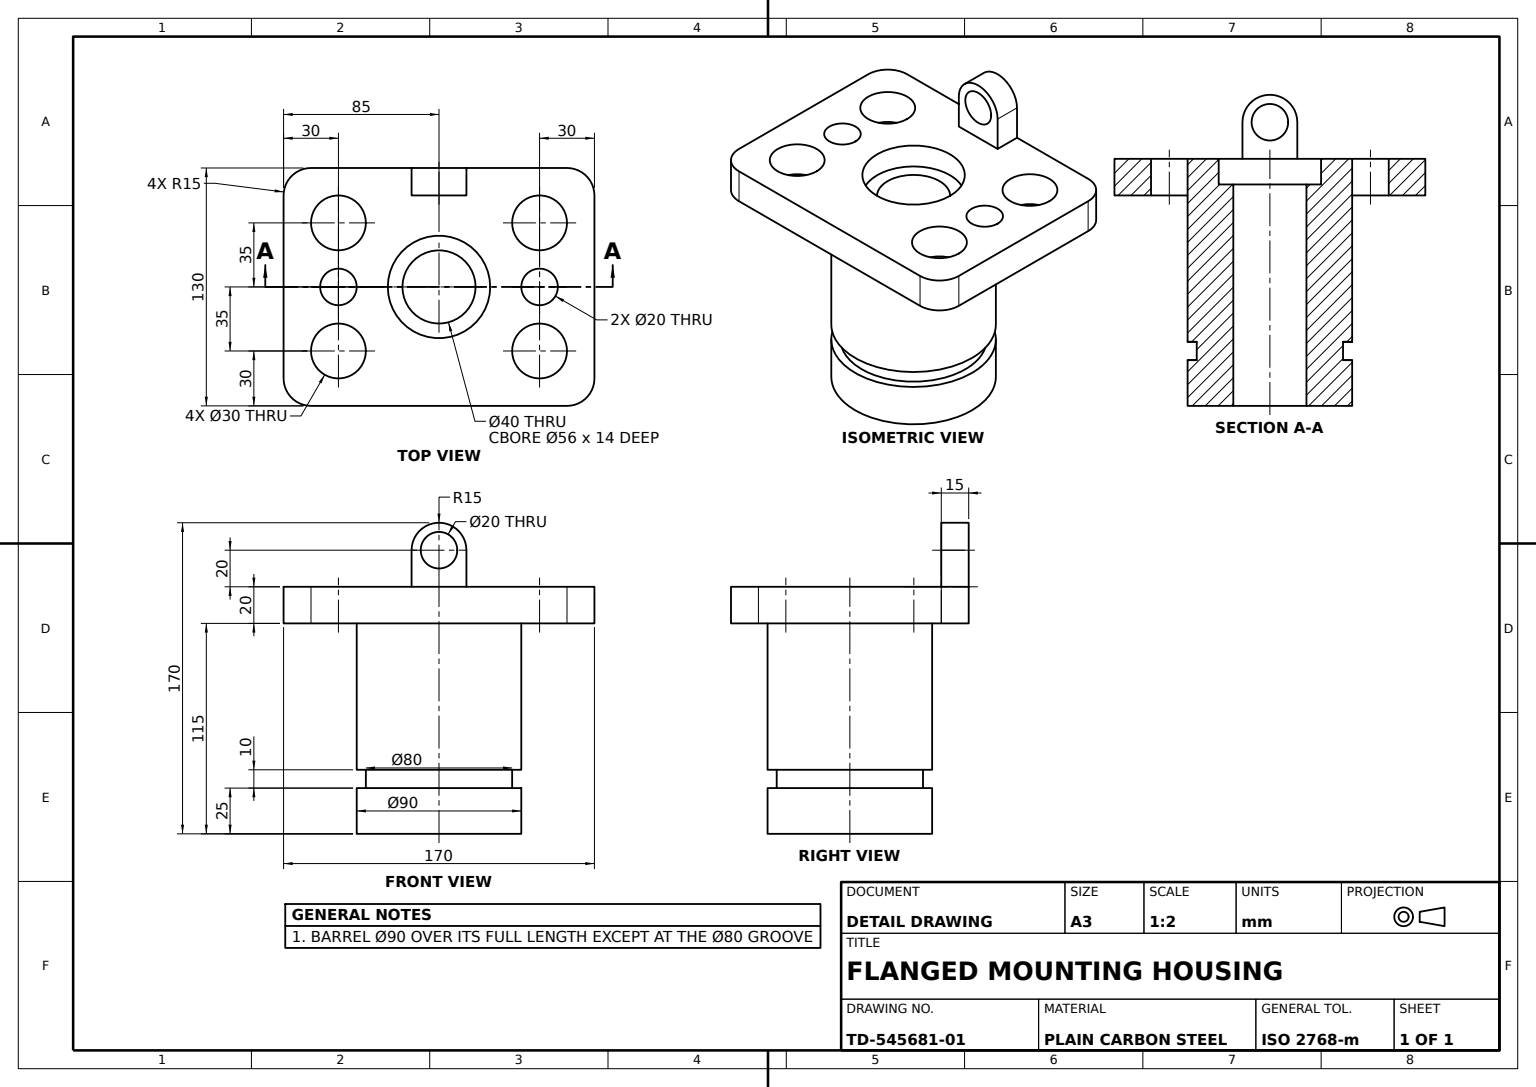
SolidWorks part; units mm, degrees
material "Plain Carbon Steel"
ref_plane "Front Plane" through (0, 0, 0) normal (0, 0, 1) x (1, 0, 0)
ref_plane "Top Plane" through (0, 0, 0) normal (0, 1, 0) x (1, 0, 0)
ref_plane "Right Plane" through (0, 0, 0) normal (1, 0, 0) x (0, 0, -1)
sketch "Barrel Sketch" plane through (0, 0, 0) normal (0, 1, 0) x (1, 0, 0)
  circle A0 centre (0, 0) radius 45
  dimension "D1" = 90
extrude "Housing Barrel Ø90" add sketch "Barrel Sketch" along normal blind 115
sketch "Mounting Flange Sketch" plane through (0, 115, 0) normal (0, 1, 0) x (1, 0, 0)
  line L1 (-65, -85) -> (65, -85)
  line L2 (-65, -85) -> (-65, 85)
  line L3 (-65, 85) -> (65, 85)
  line L4 (65, -85) -> (65, 85)
  line L5 (-65, -85) -> (65, 85) construction
  line L6 (-65, 85) -> (65, -85) construction
  point P0 (0, 0)
  dimension "D1" = 170
  dimension "D2" = 130
extrude "Mounting Flange 170x130" add sketch "Mounting Flange Sketch" along normal blind 20
sketch "Flange Holes Sketch" plane through (0, 135, 0) normal (0, 1, 0) x (1, 0, 0)
  line L0 (65, 85) -> (-65, 85) construction
  line L1 (-65, 85) -> (-65, -85) construction
  line L2 (65, -85) -> (65, 85) construction
  line L3 (-65, 0) -> (65, 0) construction
  circle A0 centre (35, 55) radius 15
  circle A1 centre (0, 55) radius 10
  circle A2 centre (-35, 55) radius 15
  circle A6 centre (-35, -55) radius 15
  circle A7 centre (0, -55) radius 10
  circle A8 centre (35, -55) radius 15
  dimension "D1" = 30
  dimension "D2" = 30
  dimension "D6" = 20
  dimension "D7" = 30
  dimension "D8" = 30
  dimension "D9" = 30
  dimension "D10" = 30
  dimension "D11" = 35
  dimension "D12" = 30
extrude "Flange Mounting Holes" cut sketch "Flange Holes Sketch" against normal blind 20
sketch "Counterbore Sketch" plane through (0, 135, 0) normal (0, 1, 0) x (1, 0, 0)
  circle A0 centre (0, 0) radius 28
  dimension "D1" = 56
extrude "Counterbore Ø56" cut sketch "Counterbore Sketch" against normal blind 14
sketch "Bore Sketch" plane through (0, 121, 0) normal (0, 1, 0) x (1, 0, 0)
  circle A0 centre (0, 0) radius 20
  dimension "D1" = 40
extrude "Bore Ø40" cut sketch "Bore Sketch" against normal through all
ref_plane "Plane2" through (0, 0, 0) normal (0, 0, 1) x (1, 0, 0)
sketch "Barrel Groove Sketch" plane through (0, 0, 0) normal (0, 0, 1) x (1, 0, 0)
  line L0 (0, 25) -> (0, 35) construction
  line L1 (0, 25) -> (-45, 25)
  line L2 (-45, 115) -> (-45, 0) construction
  line L3 (-45, 25) -> (-45, 35)
  line L4 (-45, 35) -> (0, 35)
  line L7 (0, 25) -> (0, 35)
  dimension "D1" = 45
  dimension "D2" = 10
  dimension "D3" = 25
revolve "Barrel Groove" cut sketch "Barrel Groove Sketch" angle 360 about L0
sketch "Groove Ring Sketch" plane through (0, 0, 0) normal (0, 0, 1) x (1, 0, 0)
  line L0 (0, 25) -> (0, 35) construction
  line L1 (45, 25) -> (-45, 25) construction
  line L2 (-45, 35) -> (45, 35) construction
  line L3 (0, 35) -> (-40, 35)
  line L4 (-40, 35) -> (-40, 25)
  line L5 (-40, 25) -> (0, 25)
  line L6 (0, 25) -> (0, 35)
  dimension "D1" = 40
revolve "Groove Ring" add sketch "Groove Ring Sketch" angle 360 about L0
sketch "Lifting Lug Sketch" plane through (-65, 0, 0) normal (-1, 0, 0) x (0, 0, 1)
  line L0 (-85, 135) -> (-85, 115) construction
  line L1 (-85, 135) -> (85, 135) construction
  line L2 (-15, 155) -> (-15, 135)
  line L3 (-15, 135) -> (15, 135)
  line L4 (15, 135) -> (15, 155)
  arc A0 (15, 155) -> (-15, 155) centre (0, 155) ccw
  dimension "D1" = 30
  dimension "D2" = 85
  dimension "D3" = 20
extrude "Lifting Lug" add sketch "Lifting Lug Sketch" against normal blind 15
sketch "Lug Hole Sketch" plane through (-65, 0, 0) normal (-1, 0, 0) x (0, 0, 1)
  circle A0 centre (0, 155) radius 10
  dimension "D1" = 20
extrude "Lug Hole Ø20" cut sketch "Lug Hole Sketch" against normal blind 15
fillet "Flange Corner Fillets R15" radius 15 4 edges at (-65, 125, 85) (65, 125, 85) (-65, 125, -85) (65, 125, -85)
sketch "Bottom Recess Sketch" plane through (0, 25, 0) normal (0, -1, 0) x (1, 0, 0)
  circle A0 centre (0, 0) radius 20
  dimension "D1" = 40
extrude "Bottom Recess Ø40" cut sketch "Bottom Recess Sketch" against normal blind 15
